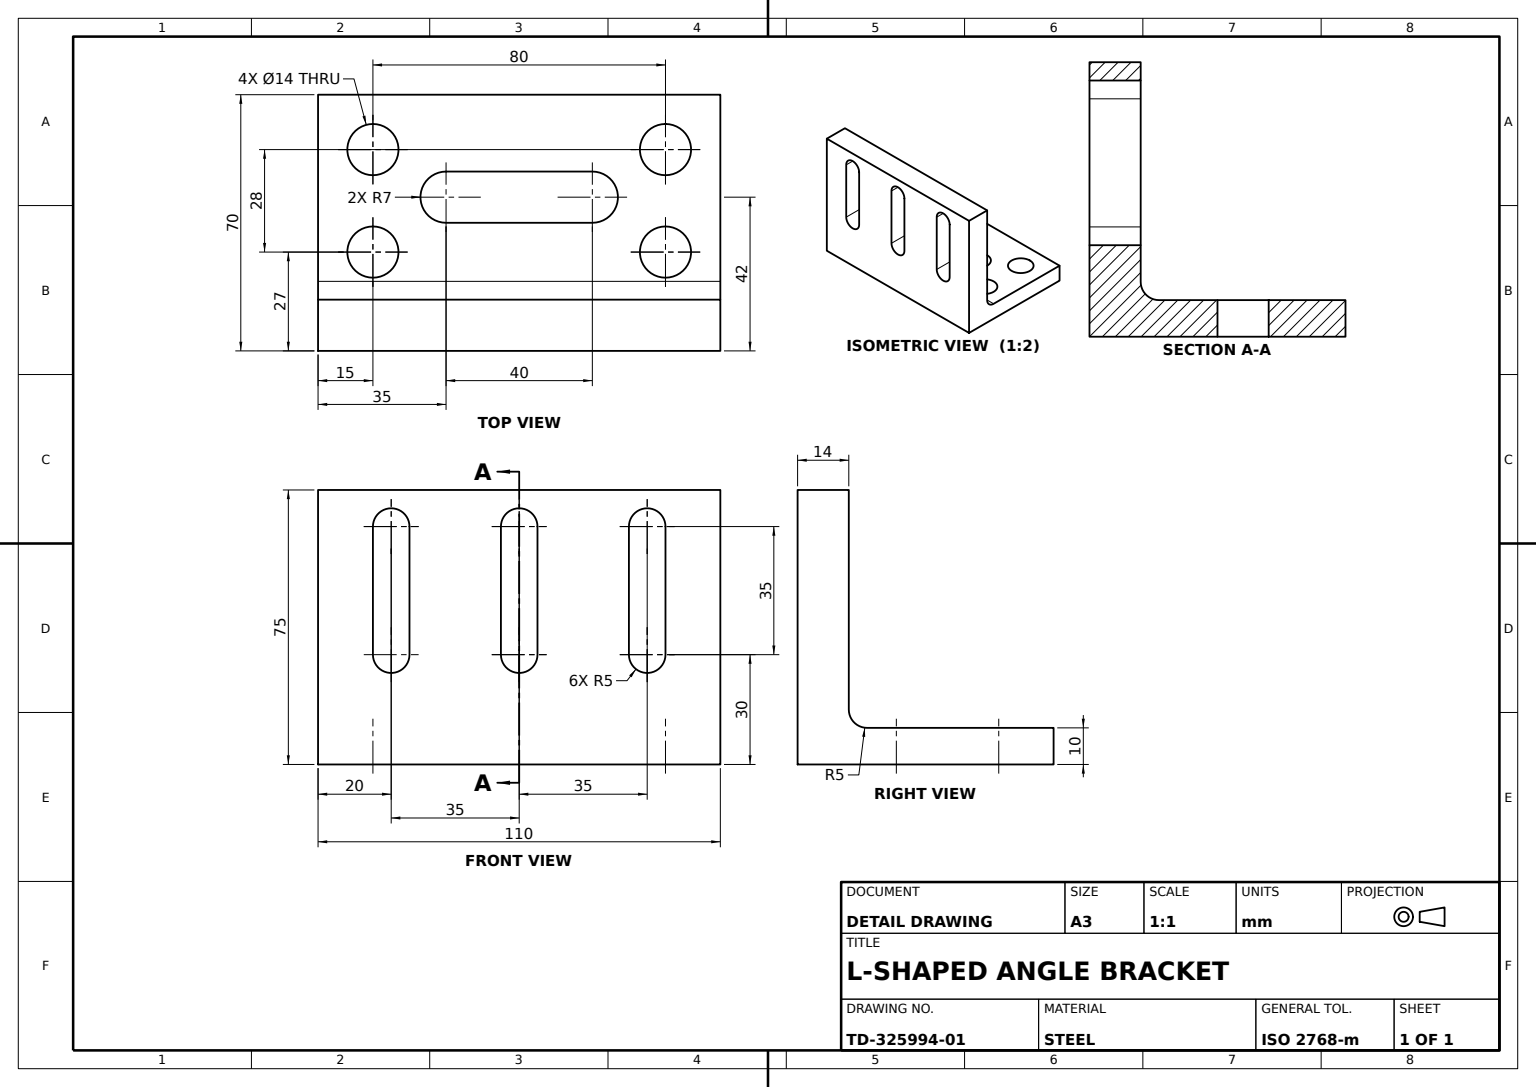
from build123d import *

# Parameters (mm, degrees)
L_BRACKET_BODY_DEPTH          = 110
VERTICAL_LEG_SLOTS_3X10_DEPTH = 110
BASE_HOLES_SKETCH_R           = 7
BASE_MOUNTING_HOLES_DEPTH     = 110
INNER_CORNER_FILLET_R5_R      = 5


with BuildPart() as part:
    # Bracket L-Profile Sketch → L-Bracket Body (new body)
    with BuildSketch(Plane(origin=(0, 0, 0), x_dir=(0, 0, -1), z_dir=(1, 0, 0))):
        Polygon((0, 0), (0, 75), (14, 75), (14, 10), (70, 10), (70, 0), align=None)
    extrude(amount=-L_BRACKET_BODY_DEPTH)

    # Vertical Leg Slots Sketch → Vertical Leg Slots 3x10 (cut)
    with BuildSketch(Plane(origin=(0, 0, -14), x_dir=(-1, 0, 0), z_dir=(0, 0, -1))):
        with BuildLine():
            Line((15, 65), (15, 30))
            ThreePointArc((15, 30), (20, 25), (25, 30))
            Line((25, 30), (25, 65))
            ThreePointArc((25, 65), (20, 70), (15, 65))
        make_face()
        with BuildLine():
            Line((50, 65), (50, 30))
            ThreePointArc((50, 30), (55, 25), (60, 30))
            Line((60, 30), (60, 65))
            ThreePointArc((60, 65), (55, 70), (50, 65))
        make_face()
        with BuildLine():
            Line((85, 65), (85, 30))
            ThreePointArc((85, 30), (90, 25), (95, 30))
            Line((95, 30), (95, 65))
            ThreePointArc((95, 65), (90, 70), (85, 65))
        make_face()
    extrude(amount=-VERTICAL_LEG_SLOTS_3X10_DEPTH, mode=Mode.SUBTRACT)

    # Base Holes Sketch → Base Mounting Holes (cut)
    with BuildSketch(Plane(origin=(0, 10, 0), x_dir=(1, 0, 0), z_dir=(0, 1, 0))):
        with Locations(Location((-95, 55, 0), (0, 0, 270))):
            Circle(BASE_HOLES_SKETCH_R)
        with Locations(Location((-15, 55, 0), (0, 0, 270))):
            Circle(BASE_HOLES_SKETCH_R)
        with Locations(Location((-15, 27, 0), (0, 0, 270))):
            Circle(BASE_HOLES_SKETCH_R)
        with Locations(Location((-95, 27, 0), (0, 0, 270))):
            Circle(BASE_HOLES_SKETCH_R)
        with BuildLine():
            Line((-75, 49), (-35, 49))
            ThreePointArc((-35, 49), (-28, 42), (-35, 35))
            Line((-35, 35), (-75, 35))
            ThreePointArc((-75, 35), (-82, 42), (-75, 49))
        make_face()
    extrude(amount=-BASE_MOUNTING_HOLES_DEPTH, mode=Mode.SUBTRACT)

    # Inner Corner Fillet R5
    inner_corner_fillet_r5_edges = [part.edges().sort_by_distance(p)[0] for p in [
        (-55, 10, -14),
    ]]
    fillet(inner_corner_fillet_r5_edges, radius=INNER_CORNER_FILLET_R5_R)


solid = part.part
